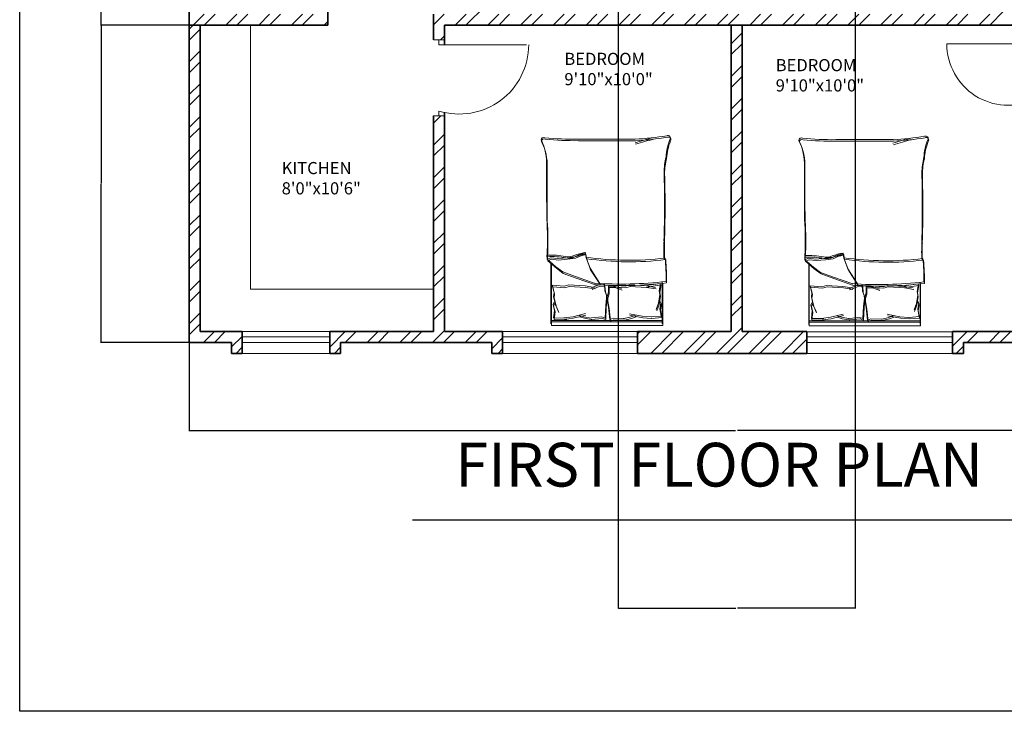
# Model space of a CAD drawing. Units: inches. Extents: x 1570 to 2186, y 1575 to 2421.
# Tile 1 of 10: x 1570 to 1975, y 1575 to 1859. Entities that reach past the tile are written whole.
import ezdxf

# ---------------------------------------------------------------- set-up
doc = ezdxf.new("R2010")
doc.units = ezdxf.units.IN
for name, color, linetype, lineweight in [('A-ANNO-DIMS', 2, 'Continuous', 18), ('A-ANNO-TTLB', 7, 'Continuous', 25), ('A-AREA-IDEN', 7, 'Continuous', 18), ('A-DOOR', 201, 'Continuous', 18), ('A-FLOR-CASE', 7, 'Continuous', 18), ('A-FURN', 8, 'Continuous', 13), ('A-GLAZ', 150, 'Continuous', 18), ('A-WALL', 7, 'Continuous', 35), ('A-WALL-PATT', 252, 'Continuous', 13)]:
    doc.layers.add(name, color=color, linetype=linetype, lineweight=lineweight)
doc.styles.get("Standard").update_dxf_attribs({"font": 'arial.ttf'})
doc.dimstyles.get("Standard").update_dxf_attribs({"dimtxt": 0.18, "dimasz": 0.18, "dimexe": 0.18, "dimexo": 0.0625, "dimgap": 0.09, "dimtad": 0, "dimtih": 1, "dimtoh": 1, "dimdec": 4, "dimzin": 0, "dimdsep": 46, "dimtxsty": 'Standard', "dimcen": 0.09, "dimadec": 0, "dimazin": 0, "dimtfac": 1, "dimtdec": 4, "dimtofl": 0, "dimtmove": 0, "dimatfit": 3, "dimfxl": 1, "dimtolj": 1, "dimtzin": 0, "dimarcsym": 0})

# ---------------------------------------------------------------- blocks, each defined once
blk = doc.blocks.new('BED-DOUBLE')
for p, q in [((3.33, 60.74), (3.33, 78.1)), ((3.33, 60.74), (3.33, 78.1)), ((3.33, 78.1), (49.16, 78.1)), ((3.55, 60.12), (3.55, 77.49)), ((3.55, 60.12), (3.55, 77.49)), ((49.16, 78.1), (49.16, 52.58)), ((49.16, 78.1), (49.16, 52.58)), ((49.38, 77.49), (49.38, 51.97)), ((49.38, 77.49), (49.38, 51.97)), ((3.33, 76.63), (49.16, 76.63)), ((3.33, 76.63), (49.16, 76.63)), ((3.55, 76.02), (49.38, 76.02)), ((3.55, 76.02), (49.38, 76.02)), ((3.74, 74.9), (7.84, 75.22)), ((3.74, 74.9), (7.84, 75.22)), ((3.74, 74.92), (4.29, 71.87)), ((3.74, 74.92), (4.29, 71.87)), ((3.95, 74.31), (4.51, 71.26)), ((3.95, 74.31), (4.51, 71.26)), ((3.96, 74.29), (8.06, 74.6)), ((3.96, 74.29), (8.06, 74.6)), ((7.84, 75.22), (7.95, 75.2)), ((7.84, 75.22), (7.95, 75.2)), ((7.95, 75.2), (11.61, 74.92)), ((7.95, 75.2), (11.61, 74.92)), ((8.06, 74.6), (8.16, 74.59)), ((8.06, 74.6), (8.16, 74.59)), ((8.16, 74.59), (11.83, 74.31)), ((8.16, 74.59), (11.83, 74.31)), ((11.61, 74.92), (16.88, 73.95)), ((11.61, 74.92), (16.88, 73.95)), ((11.83, 74.31), (17.1, 73.34)), ((11.83, 74.31), (17.1, 73.34)), ((14.25, 74.51), (16.19, 75.2)), ((14.25, 74.51), (16.19, 75.2)), ((14.46, 73.89), (16.41, 74.59)), ((14.47, 73.89), (16.41, 74.59)), ((16.19, 75.2), (18.96, 75.89)), ((16.19, 75.2), (18.96, 75.89)), ((16.41, 74.59), (19.18, 75.28)), ((16.41, 74.59), (19.18, 75.28)), ((18.96, 75.89), (19.27, 75.89)), ((18.96, 75.89), (19.27, 75.89)), ((19.18, 75.28), (19.49, 75.28)), ((19.18, 75.28), (19.49, 75.28)), ((19.27, 75.89), (23.53, 75.76)), ((19.27, 75.89), (23.53, 75.76)), ((19.49, 75.28), (23.75, 75.14)), ((19.49, 75.28), (23.75, 75.14)), ((23.53, 75.76), (24.92, 76.31)), ((23.53, 75.76), (24.92, 76.31)), ((23.75, 75.14), (25.14, 75.7)), ((23.75, 75.14), (25.14, 75.7)), ((24.92, 76.31), (25.47, 71.18)), ((24.92, 76.31), (25.47, 71.18)), ((25.14, 75.7), (25.69, 70.57)), ((25.14, 75.7), (25.69, 70.57)), ((26.83, 75.71), (26.6, 70.56)), ((26.83, 75.71), (26.6, 70.56)), ((27.05, 75.1), (26.82, 69.95)), ((27.05, 75.1), (26.82, 69.95)), ((28.25, 75.25), (26.83, 75.71)), ((28.25, 75.25), (26.83, 75.71)), ((28.47, 74.63), (27.05, 75.1)), ((28.47, 74.63), (27.05, 75.1)), ((32.49, 75.65), (28.25, 75.25)), ((32.49, 75.65), (28.25, 75.25)), ((32.71, 75.04), (28.47, 74.63)), ((32.71, 75.04), (28.47, 74.63)), ((32.8, 75.67), (32.49, 75.65)), ((32.8, 75.67), (32.49, 75.65)), ((33.02, 75.06), (32.71, 75.04)), ((33.02, 75.06), (32.71, 75.04)), ((35.61, 75.15), (32.8, 75.67)), ((35.61, 75.15), (32.8, 75.67)), ((35.83, 74.54), (33.02, 75.06)), ((35.83, 74.54), (33.02, 75.06)), ((40.2, 75.16), (35, 73.86)), ((40.2, 75.16), (35, 73.86)), ((40.42, 74.55), (35.22, 73.25)), ((40.41, 74.55), (35.22, 73.25)), ((37.59, 74.58), (35.61, 75.15)), ((37.59, 74.58), (35.61, 75.15)), ((37.81, 73.97), (35.83, 74.54)), ((37.81, 73.97), (35.83, 74.54)), ((43.84, 75.67), (40.2, 75.16)), ((43.84, 75.67), (40.2, 75.16)), ((44.06, 75.05), (40.41, 74.55)), ((44.06, 75.05), (40.42, 74.55)), ((48.06, 75.65), (42.88, 75.74)), ((42.88, 75.74), (43.84, 75.67)), ((48.06, 75.65), (42.88, 75.74)), ((42.88, 75.74), (43.84, 75.67)), ((48.28, 75.04), (43.1, 75.13)), ((43.1, 75.13), (44.06, 75.05)), ((48.28, 75.04), (43.1, 75.13)), ((43.1, 75.13), (44.06, 75.05)), ((48.06, 75.65), (47.69, 72.57)), ((48.06, 75.65), (47.69, 72.57)), ((48.28, 75.04), (47.91, 71.96)), ((48.28, 75.04), (47.91, 71.96)), ((4.29, 71.87), (3.87, 69.38)), ((4.29, 71.87), (3.87, 69.38)), ((3.87, 69.38), (4.43, 68.41)), ((3.87, 69.38), (4.43, 68.41)), ((4.51, 71.26), (4.09, 68.76)), ((4.51, 71.26), (4.09, 68.76)), ((4.29, 66.05), (4.84, 69.52)), ((4.29, 66.05), (4.84, 69.52)), ((4.51, 65.44), (5.06, 68.9)), ((4.51, 65.44), (5.06, 68.9)), ((4.84, 69.52), (5.81, 72.15)), ((4.84, 69.52), (5.81, 72.15)), ((5.06, 68.9), (6.03, 71.54)), ((5.06, 68.9), (6.03, 71.54)), ((25.47, 71.18), (26.03, 68.13)), ((25.47, 71.18), (26.03, 68.13)), ((25.69, 70.57), (26.25, 67.52)), ((25.69, 70.57), (26.25, 67.52)), ((26.6, 70.56), (26.23, 67.48)), ((26.6, 70.56), (26.23, 67.48)), ((26.82, 69.95), (26.45, 66.87)), ((26.82, 69.95), (26.45, 66.87)), ((47.29, 70.18), (46.15, 72.75)), ((47.29, 70.18), (46.16, 72.75)), ((47.51, 69.57), (46.37, 72.14)), ((47.51, 69.57), (46.37, 72.14)), ((48.06, 66.76), (47.29, 70.18)), ((48.06, 66.76), (47.29, 70.18)), ((48.28, 66.15), (47.51, 69.57)), ((48.28, 66.15), (47.51, 69.57)), ((47.69, 72.57), (48.27, 70.11)), ((47.69, 72.57), (48.26, 70.11)), ((48.27, 70.11), (47.77, 69.1)), ((48.26, 70.11), (47.77, 69.1)), ((47.91, 71.96), (48.48, 69.49)), ((47.91, 71.96), (48.48, 69.49)), ((48.48, 69.49), (47.99, 68.49)), ((48.48, 69.49), (47.99, 68.49)), ((4.09, 68.76), (4.65, 67.79)), ((4.09, 68.76), (4.65, 67.79)), ((4.57, 64.52), (4.29, 66.05)), ((4.57, 64.52), (4.29, 66.05)), ((4.79, 63.91), (4.51, 65.44)), ((4.79, 63.91), (4.51, 65.44)), ((26.03, 66.88), (25.47, 65.08)), ((26.03, 66.88), (25.47, 65.08)), ((25.47, 65.08), (25.47, 62.51)), ((25.47, 65.08), (25.47, 62.51)), ((26.25, 66.27), (25.69, 64.47)), ((26.25, 66.27), (25.69, 64.47)), ((26.03, 68.13), (26.03, 66.88)), ((26.03, 68.13), (26.03, 66.88)), ((26.23, 67.48), (26.31, 66.23)), ((26.23, 67.48), (26.31, 66.23)), ((26.25, 67.52), (26.25, 66.27)), ((26.25, 67.52), (26.25, 66.27)), ((26.31, 66.23), (26.98, 64.47)), ((26.31, 66.23), (26.98, 64.47)), ((26.45, 66.87), (26.53, 65.62)), ((26.45, 66.87), (26.53, 65.62)), ((26.53, 65.62), (27.2, 63.86)), ((26.53, 65.62), (27.2, 63.86)), ((47.88, 65.22), (48.06, 66.76)), ((47.88, 65.22), (48.06, 66.76)), ((48.62, 62.21), (47.88, 65.22)), ((48.62, 62.21), (47.88, 65.22)), ((48.09, 64.61), (48.28, 66.15)), ((48.1, 64.61), (48.28, 66.15)), ((4.01, 61.47), (4.57, 64.52)), ((4.01, 61.47), (4.57, 64.52)), ((8.9, 62.17), (4.01, 61.47)), ((8.9, 62.17), (4.01, 61.47)), ((4.23, 60.86), (4.79, 63.91)), ((4.23, 60.86), (4.79, 63.91)), ((9.12, 61.55), (4.23, 60.86)), ((9.12, 61.55), (4.23, 60.86)), ((6.12, 63.12), (9.99, 62.48)), ((6.12, 63.12), (9.99, 62.48)), ((6.34, 62.5), (10.21, 61.86)), ((6.34, 62.5), (10.21, 61.86)), ((9.99, 62.48), (8.9, 62.17)), ((9.99, 62.48), (8.9, 62.17)), ((10.21, 61.86), (9.12, 61.55)), ((10.21, 61.86), (9.12, 61.55)), ((9.99, 62.48), (16.71, 62.06)), ((9.99, 62.48), (16.71, 62.06)), ((10.21, 61.86), (16.93, 61.45)), ((10.21, 61.86), (16.93, 61.45)), ((16.71, 62.06), (18.59, 62.6)), ((16.71, 62.06), (18.59, 62.6)), ((16.93, 61.45), (18.81, 61.98)), ((16.93, 61.45), (18.81, 61.98)), ((18.59, 62.6), (23.51, 62.21)), ((18.59, 62.6), (23.51, 62.21)), ((18.81, 61.98), (23.73, 61.6)), ((18.81, 61.98), (23.73, 61.6)), ((23.12, 62.51), (20.1, 63.55)), ((23.12, 62.51), (20.1, 63.55)), ((23.33, 61.89), (20.32, 62.94)), ((23.33, 61.89), (20.32, 62.94)), ((25.47, 62.51), (23.12, 62.51)), ((25.47, 62.51), (23.12, 62.51)), ((25.69, 61.89), (23.33, 61.89)), ((25.69, 61.89), (23.33, 61.89)), ((25.69, 64.47), (25.69, 61.89)), ((25.69, 64.47), (25.69, 61.89)), ((26.98, 64.47), (27.14, 61.9)), ((26.98, 64.47), (27.14, 61.9)), ((27.14, 61.9), (29.49, 62.05)), ((27.14, 61.9), (29.49, 62.05)), ((27.2, 63.86), (27.36, 61.29)), ((27.2, 63.86), (27.36, 61.29)), ((27.36, 61.29), (29.71, 61.44)), ((27.36, 61.29), (29.71, 61.44)), ((29.02, 61.43), (33.04, 55.21)), ((29.02, 61.43), (33.04, 55.21)), ((29.24, 60.82), (33.26, 54.59)), ((29.24, 60.82), (33.26, 54.59)), ((29.49, 62.05), (32.43, 63.28)), ((29.49, 62.05), (32.43, 63.28)), ((29.71, 61.44), (32.65, 62.67)), ((29.71, 61.44), (32.65, 62.67)), ((38.98, 58.62), (30.98, 61.43)), ((38.98, 58.62), (30.98, 61.43)), ((39.2, 58.01), (31.2, 60.82)), ((39.2, 58.01), (31.2, 60.82)), ((31.23, 63.12), (35.1, 62.48)), ((31.23, 63.12), (35.1, 62.48)), ((31.45, 62.5), (35.31, 61.86)), ((31.45, 62.5), (35.31, 61.86)), ((35.1, 62.48), (41.82, 62.06)), ((35.1, 62.48), (41.82, 62.06)), ((35.31, 61.86), (42.04, 61.45)), ((35.31, 61.86), (42.04, 61.45)), ((41.82, 62.06), (43.7, 62.6)), ((41.82, 62.06), (43.7, 62.6)), ((42.04, 61.45), (43.92, 61.98)), ((42.04, 61.45), (43.92, 61.98)), ((43.7, 62.6), (48.62, 62.21)), ((43.7, 62.6), (48.62, 62.21)), ((43.92, 61.98), (48.84, 61.6)), ((43.92, 61.98), (48.84, 61.6)), ((48.84, 61.6), (48.09, 64.61)), ((48.84, 61.6), (48.1, 64.61)), ((44.32, 56.69), (38.98, 58.62)), ((44.32, 56.69), (38.98, 58.62)), ((44.54, 56.08), (39.2, 58.01)), ((44.54, 56.08), (39.2, 58.01)), ((33.04, 55.21), (34.67, 50.9)), ((33.04, 55.21), (34.67, 50.9)), ((33.26, 54.59), (34.89, 50.29)), ((33.26, 54.59), (34.89, 50.29)), ((47.15, 54.61), (44.32, 56.69)), ((47.15, 54.61), (44.32, 56.69)), ((47.37, 54), (44.54, 56.08)), ((47.37, 54), (44.54, 56.08)), ((50.7, 51.5), (47.15, 54.61)), ((50.7, 51.5), (47.15, 54.61)), ((50.92, 50.88), (47.37, 54)), ((50.92, 50.88), (47.37, 54)), ((34.67, 50.9), (34.97, 48.97)), ((34.67, 50.9), (34.97, 48.97)), ((34.89, 50.29), (35.19, 48.36)), ((34.89, 50.29), (35.19, 48.36)), ((34.97, 48.97), (37.34, 49.57)), ((34.97, 48.97), (37.34, 49.57)), ((35.19, 48.36), (37.56, 48.95)), ((35.19, 48.36), (37.56, 48.95)), ((37.34, 49.57), (39.27, 50.46)), ((37.34, 49.57), (39.27, 50.46)), ((37.56, 48.95), (39.49, 49.84)), ((37.56, 48.95), (39.49, 49.84)), ((39.27, 50.46), (42.54, 50.9)), ((39.27, 50.46), (42.54, 50.9)), ((39.49, 49.84), (42.76, 50.29)), ((39.49, 49.84), (42.76, 50.29)), ((42.54, 50.9), (46.26, 51.2)), ((42.54, 50.9), (46.26, 51.2)), ((42.76, 50.29), (46.47, 50.59)), ((42.76, 50.29), (46.47, 50.59)), ((46.26, 51.2), (49.23, 50.9)), ((46.26, 51.2), (49.23, 50.9)), ((46.47, 50.59), (49.45, 50.29)), ((46.47, 50.59), (49.44, 50.29)), ((49.23, 50.9), (50.7, 51.5)), ((49.23, 50.9), (50.7, 51.5)), ((49.44, 50.29), (50.92, 50.88)), ((49.45, 50.29), (50.92, 50.88)), ((50.78, 49.82), (50.7, 51.5, 3.71)), ((50.78, 49.82), (50.7, 51.5, 3.71)), ((51, 49.21), (50.92, 50.88, 3.71)), ((51, 49.21), (50.92, 50.88, 3.71)), ((14.45, 2.11), (38.05, 2.11)), ((14.45, 2.11), (38.05, 2.11)), ((14.66, 1.49), (38.27, 1.49)), ((14.67, 1.49), (38.27, 1.49))]:
    blk.add_line(p, q)
for centre, radius, start, end in [((20.48, -96.48), 158.2, 86.0865, 96.7821), ((20.48, -96.48), 158.2, 86.0865, 96.7821), ((20.7, -97.1), 158.2, 86.0865, 96.7821), ((20.7, -97.1), 158.2, 86.0865, 96.7821), ((81.67, 58.83), 79.89, 178.7218, 185.604), ((81.67, 58.83), 79.89, 178.7218, 185.604), ((81.89, 58.22), 79.89, 178.7218, 185.604), ((81.89, 58.22), 79.89, 178.7218, 185.604), ((17.03, -71.8), 123.73, 81.7845, 96.9006), ((17.03, -71.8), 123.73, 81.7845, 96.9006), ((17.25, -72.42), 123.73, 81.7845, 96.9006), ((17.25, -72.42), 123.73, 81.7845, 96.9006), ((-160.45, 48.21), 163.13, 358.4762, 1.0082), ((-160.45, 48.21), 163.13, 358.4762, 1.0082), ((-160.23, 47.59), 163.13, 358.4762, 1.0082), ((-160.23, 47.59), 163.13, 358.4762, 1.0082), ((35.13, 48.91), 0.177, 160.2464, 271.1377), ((35.13, 48.91), 0.177, 160.2464, 271.1377), ((29.88, 76.68), 28.44, 280.6617, 289.8806), ((29.88, 76.68), 28.44, 280.6617, 289.8806), ((30.1, 76.07), 28.44, 280.6617, 289.8806), ((30.1, 76.07), 28.44, 280.6617, 289.8806), ((41.95, 44.48), 5.97, 78.6608, 113.7384), ((41.95, 44.48), 5.97, 78.6608, 113.7384), ((42.17, 43.86), 5.97, 78.6608, 113.7384), ((42.17, 43.86), 5.97, 78.6608, 113.7384), ((49.22, 84.49), 34.7, 259.8763, 272.5657), ((49.22, 84.49), 34.7, 259.8763, 272.5657), ((49.44, 83.87), 34.7, 259.8763, 272.5657), ((49.44, 83.87), 34.7, 259.8763, 272.5657), ((174.79, 43.28), 124.19, 176.9791, 183.8365), ((174.79, 43.28), 124.19, 176.9791, 183.8365), ((175.01, 42.66), 124.19, 176.9791, 183.8365), ((175.01, 42.66), 124.19, 176.9791, 183.8365), ((35.35, 48.3), 0.177, 160.2464, 271.1377), ((35.35, 48.3), 0.177, 160.2464, 271.1377), ((464.94, 29.56), 462.53, 178.2277, 181.7185), ((464.94, 29.56), 462.53, 178.2277, 181.7185), ((465.16, 28.95), 462.53, 178.2277, 181.7185), ((465.16, 28.95), 462.53, 178.2277, 181.7185), ((-4323.86, 13.06), 4374.8, 0.00217, 0.28689), ((-4323.86, 13.06), 4374.8, 0.00217, 0.28689), ((-4323.64, 12.45), 4374.8, 0.00217, 0.28689), ((-4323.64, 12.45), 4374.8, 0.00217, 0.28689), ((-25.8, 16.23), 28.42, 346.0648, 358.9113), ((-25.8, 16.23), 28.42, 346.0648, 358.9113), ((-25.58, 15.62), 28.42, 346.0648, 358.9113), ((-25.58, 15.62), 28.42, 346.0648, 358.9113), ((73.03, 12.25), 22.12, 177.4714, 206.4681), ((73.03, 12.25), 22.12, 177.4714, 206.4681), ((73.25, 11.64), 22.12, 177.4714, 206.4681), ((73.25, 11.64), 22.12, 177.4714, 206.4681), ((-20.77, 10.71), 22.6, 337.9751, 356.652), ((-20.77, 10.71), 22.6, 337.9751, 356.652), ((-20.55, 10.1), 22.6, 337.9751, 356.652), ((-20.55, 10.1), 22.6, 337.9751, 356.652), ((1.04, 1.65), 1.04, 146.1736, 293.4781), ((1.04, 1.65), 1.04, 146.1736, 293.4781), ((1.26, 1.04), 1.04, 146.1736, 293.4781), ((1.26, 1.04), 1.04, 146.1736, 293.4781), ((20.55, -114.5), 116.77, 92.9958, 99.4091), ((20.55, -114.5), 116.77, 92.9958, 99.4091), ((20.77, -115.11), 116.77, 92.9958, 99.4091), ((20.77, -115.11), 116.77, 92.9958, 99.4091), ((-16.52, 100.84), 102.09, 283.3832, 287.7053), ((-16.52, 100.84), 102.09, 283.3832, 287.7053), ((-16.3, 100.23), 102.09, 283.3832, 287.7053), ((-16.3, 100.23), 102.09, 283.3832, 287.7053), ((39.46, -125.47), 127.58, 84.4998, 90.6351), ((39.46, -125.47), 127.58, 84.4998, 90.6351), ((39.68, -126.08), 127.58, 84.4998, 90.6351), ((39.68, -126.08), 127.58, 84.4998, 90.6351), ((52.18, 2.47), 1.06, 242.6588, 356.02), ((52.18, 2.47), 1.06, 242.6588, 356.02), ((52.4, 1.85), 1.06, 242.6588, 356.02), ((52.4, 1.85), 1.06, 242.6588, 356.02)]:
    blk.add_arc(centre, radius, start, end)
blk = doc.blocks.new('*D31')
at = {"layer": 'A-ANNO-DIMS', "color": 0, "lineweight": -2, "transparency": 16777216}
for p, q in [((1639.59, 1726.19), (1639.59, 1689.77)), ((2090.09, 1726.19), (2090.09, 1689.77)), ((1639.77, 1689.95), (1864.44, 1689.95)), ((2089.91, 1689.95), (1865.24, 1689.95))]:
    blk.add_line(p, q, dxfattribs=at)
at = {"layer": 'A-ANNO-DIMS', "color": 0, "transparency": 16777216}
for points in [[(1639.77, 1689.98), (1639.77, 1689.92), (1639.59, 1689.95)], [(2089.91, 1689.98), (2089.91, 1689.92), (2090.09, 1689.95)]]:
    blk.add_solid(points, dxfattribs=at)
at = {"layer": 'Defpoints', "color": 0, "transparency": 16777216}
for p in [(1639.59, 1726.25), (2090.09, 1726.25), (1639.59, 1689.95)]:
    blk.add_point(p, dxfattribs=at)
at = {"layer": 'A-ANNO-DIMS', "color": 0, "transparency": 16777216, "insert": (1864.84, 1689.95), "char_height": 0.18, "attachment_point": 5}
blk.add_mtext('\\A1;450.5', dxfattribs=at)
blk = doc.blocks.new('*D33')
at = {"layer": 'A-ANNO-DIMS', "color": 0, "lineweight": -2, "transparency": 16777216}
for p, q in [((1639.53, 1856.75), (1603.11, 1856.75)), ((1603.29, 1856.57), (1603.29, 1791.68)), ((1603.29, 1726.43), (1603.29, 1791.32)), ((1639.53, 1726.25), (1603.11, 1726.25))]:
    blk.add_line(p, q, dxfattribs=at)
at = {"layer": 'A-ANNO-DIMS', "color": 0, "transparency": 16777216}
for points in [[(1603.26, 1856.57), (1603.32, 1856.57), (1603.29, 1856.75)], [(1603.26, 1726.43), (1603.32, 1726.43), (1603.29, 1726.25)]]:
    blk.add_solid(points, dxfattribs=at)
at = {"layer": 'Defpoints', "color": 0, "transparency": 16777216}
for p in [(1603.29, 1856.75), (1639.59, 1856.75), (1639.59, 1726.25)]:
    blk.add_point(p, dxfattribs=at)
at = {"layer": 'A-ANNO-DIMS', "color": 0, "transparency": 16777216, "insert": (1603.29, 1791.5), "char_height": 0.18, "attachment_point": 5}
blk.add_mtext('\\A1;130.5', dxfattribs=at)
blk = doc.blocks.new('*D34')
at = {"layer": 'A-ANNO-DIMS', "color": 0, "lineweight": -2, "transparency": 16777216}
for p, q in [((1639.53, 1913.75), (1603.11, 1913.75)), ((1603.29, 1913.57), (1603.29, 1885.43)), ((1603.29, 1856.93), (1603.29, 1885.07)), ((1639.53, 1856.75), (1603.11, 1856.75))]:
    blk.add_line(p, q, dxfattribs=at)
at = {"layer": 'A-ANNO-DIMS', "color": 0, "transparency": 16777216}
for points in [[(1603.26, 1913.57), (1603.32, 1913.57), (1603.29, 1913.75)], [(1603.26, 1856.93), (1603.32, 1856.93), (1603.29, 1856.75)]]:
    blk.add_solid(points, dxfattribs=at)
at = {"layer": 'Defpoints', "color": 0, "transparency": 16777216}
for p in [(1603.29, 1913.75), (1639.59, 1913.75), (1639.59, 1856.75)]:
    blk.add_point(p, dxfattribs=at)
at = {"layer": 'A-ANNO-DIMS', "color": 0, "transparency": 16777216, "insert": (1603.29, 1885.25), "char_height": 0.18, "attachment_point": 5}
blk.add_mtext('\\A1;57', dxfattribs=at)
blk = doc.blocks.new('*D39')
at = {"layer": 'A-ANNO-DIMS', "color": 0, "lineweight": -2, "transparency": 16777216}
for p, q in [((1816.09, 2097.8), (1816.09, 1616.73)), ((1913.59, 2097.8), (1913.59, 1616.73)), ((1816.27, 1616.91), (1864.51, 1616.91)), ((1913.41, 1616.91), (1865.16, 1616.91))]:
    blk.add_line(p, q, dxfattribs=at)
at = {"layer": 'A-ANNO-DIMS', "color": 0, "transparency": 16777216}
for points in [[(1816.27, 1616.94), (1816.27, 1616.88), (1816.09, 1616.91)], [(1913.41, 1616.94), (1913.41, 1616.88), (1913.59, 1616.91)]]:
    blk.add_solid(points, dxfattribs=at)
at = {"layer": 'Defpoints', "color": 0, "transparency": 16777216}
for p in [(1816.09, 2097.86), (1913.59, 2097.86), (1913.59, 1616.91)]:
    blk.add_point(p, dxfattribs=at)
at = {"layer": 'A-ANNO-DIMS', "color": 0, "transparency": 16777216, "insert": (1864.84, 1616.91), "char_height": 0.18, "attachment_point": 5}
blk.add_mtext('\\A1;97.5', dxfattribs=at)

msp = doc.modelspace()

# ---------------------------------------------------------------- hatches: boundary and pattern name
at = {"layer": 'A-WALL-PATT'}
h = msp.add_hatch(dxfattribs=at)
h.set_pattern_fill('ANSI32', color=256)
h.paths.add_polyline_path([(1762.0975, 2362.1492), (1757.5975, 2362.1492), (1757.5975, 2357.6492), (1709.1163, 2357.6492), (1709.1163, 2362.1492), (1704.6163, 2362.1492), (1704.6163, 2353.1492), (1740.0886, 2353.1492), (1740.0886, 2261.8115), (1744.5886, 2261.8115), (1744.5886, 2353.1492), (1762.0975, 2353.1492)])
h.paths.add_polyline_path([(1890.2592, 2362.1492), (1885.7592, 2362.1492), (1826.5975, 2362.1492), (1822.0975, 2362.1492), (1822.0975, 2353.1492), (1862.5886, 2353.1492), (1862.5886, 2227.1492), (1744.5886, 2227.1492), (1744.5886, 2229.5389), (1742.3386, 2229.5389), (1740.0886, 2229.5389), (1740.0886, 2222.6492), (1744.5886, 2222.6492), (1756.186, 2222.6492), (1756.186, 2216.3571), (1760.686, 2216.3571), (1760.686, 2222.6492), (1832.686, 2222.6492), (1832.686, 2212.5994), (1837.186, 2212.5994), (1837.186, 2222.6492), (1893.186, 2222.6492), (1893.186, 2212.5994), (1897.686, 2212.5994), (1897.686, 2222.6492), (1989.5886, 2222.6492), (1989.5886, 2227.1492), (1989.5886, 2232.6585), (1987.3386, 2232.6585), (1985.0886, 2232.6585), (1985.0886, 2227.1492), (1867.0886, 2227.1492), (1867.0886, 2353.1492), (1890.2592, 2353.1492)])
h.paths.add_polyline_path([(1644.0886, 2353.1492), (1668.6163, 2353.1492), (1668.6163, 2362.1492), (1664.1163, 2362.1492), (1664.1163, 2358.9932), (1664.1163, 2357.6492), (1639.5886, 2357.6492), (1639.5886, 2213.8746), (1644.0886, 2213.8746), (1644.0886, 2222.6492), (1692.0886, 2222.6492), (1692.0886, 2215.9343), (1696.5886, 2215.9343), (1696.5886, 2222.6492), (1696.5886, 2227.1492), (1644.0886, 2227.1492)])
h.paths.add_polyline_path([(2013.0435, 2362.1492), (2008.5435, 2362.1492), (2008.5435, 2357.6492), (1954.7592, 2357.6492), (1954.7592, 2362.1492), (1950.2592, 2362.1492), (1950.2592, 2353.1492), (1985.0886, 2353.1492), (1985.0886, 2260.8534), (1989.5886, 2260.8534), (1989.5886, 2353.1492), (2013.0435, 2353.1492)])
h.paths.add_polyline_path([(2090.0886, 2357.6492), (2053.5435, 2357.6492), (2053.5435, 2362.1492), (2049.0435, 2362.1492), (2049.0435, 2353.1492), (2085.5886, 2353.1492), (2085.5886, 2227.1492), (2033.0886, 2227.1492), (2033.0886, 2222.6492), (2033.0886, 2214.4464), (2037.5886, 2214.4464), (2037.5886, 2222.6492), (2085.5886, 2222.6492), (2085.5886, 2212.4409), (2090.0886, 2212.4409)])
h.paths.add_polyline_path([(2090.0886, 2188.4409), (2087.8386, 2188.4409), (2085.5886, 2188.4409), (2085.5886, 2180.6492), (2037.5886, 2180.6492), (2037.5886, 2196.7956), (2033.0886, 2196.7956), (2033.0886, 2176.1492), (2037.5886, 2176.1492), (2045.0886, 2176.1492), (2045.0886, 2169.8988), (2049.5886, 2169.8988), (2049.5886, 2176.1492), (2085.5886, 2176.1492), (2085.5886, 2167.785), (2090.0886, 2167.785)])
h.paths.add_polyline_path([(2049.5886, 2147.4502), (2047.3386, 2147.4502), (2045.0886, 2147.4502), (2045.0886, 2124.4703), (2049.5886, 2124.4703)])
h.paths.add_polyline_path([(2090.0886, 2047.1492), (2049.5886, 2047.1492), (2049.5886, 2064.4703), (2045.0886, 2064.4703), (2045.0886, 2047.1492), (1918.0886, 2047.1492), (1918.0886, 2051.2061), (1913.5886, 2051.2061), (1913.5886, 2047.1492), (1913.5886, 2036.6872), (1918.0886, 2036.6872), (1918.0886, 2042.7492), (2045.0886, 2042.7492), (2045.0886, 2027.0686), (2049.5886, 2027.0686), (2049.5886, 2042.7492), (2090.0886, 2042.7492)])
h.paths.add_polyline_path([(1918.0886, 2005.9338), (1915.8386, 2005.9338), (1913.5886, 2005.9338), (1913.5886, 1913.7492), (1918.0886, 1913.7492)])
h.paths.add_polyline_path([(2090.0886, 1913.7492), (2049.5886, 1913.7492), (2045.0886, 1913.7492), (2033.0886, 1913.7492), (2033.0886, 1909.2492), (2033.0886, 1900.9803), (2037.5886, 1900.9803), (2037.5886, 1909.2492), (2085.5886, 1909.2492), (2085.5886, 1861.2492), (2037.5886, 1861.2492), (2037.5886, 1880.0859), (2033.0886, 1880.0859), (2033.0886, 1856.7492), (2085.5886, 1856.7492), (2085.5886, 1730.7492), (2054.2483, 1730.7492), (2054.2483, 1721.7492), (2058.7483, 1721.7492), (2058.7483, 1726.2492), (2090.0886, 1726.2492)])
h.paths.add_polyline_path([(2049.5886, 1967.0686), (2045.0886, 1967.0686), (2045.0886, 1913.7492), (2049.5886, 1913.7492)])
h.paths.add_polyline_path([(1989.5886, 1824.1695), (1987.3386, 1824.1695), (1985.0886, 1824.1695), (1985.0886, 1730.7492), (1989.5886, 1730.7492)])
h.paths.add_polyline_path([(1989.5886, 1861.2492), (1974.9963, 1861.2492), (1974.9963, 1865.9306), (1972.7463, 1865.9306), (1970.4963, 1865.9306), (1970.4963, 1861.2492), (1898.4963, 1861.2492), (1898.4963, 1874.2999), (1893.9963, 1874.2999), (1893.9963, 1861.2492), (1890.5886, 1861.2492), (1837.9963, 1861.2492), (1837.9963, 1874.3159), (1833.4963, 1874.3159), (1833.4963, 1861.2492), (1761.4963, 1861.2492), (1761.4963, 1865.0209), (1759.2463, 1865.0209), (1756.9963, 1865.0209), (1756.9963, 1861.2492), (1740.0886, 1861.2492), (1740.0886, 1856.7492), (1740.0886, 1850.7206), (1744.5886, 1850.7206), (1744.5886, 1856.7492), (1985.0886, 1856.7492), (1985.0886, 1851.0804), (1989.5886, 1851.0804), (1989.5886, 1856.7492)])
h.paths.add_polyline_path([(1989.5886, 1913.7492), (1740.0886, 1913.7492), (1740.0886, 1909.2492), (1756.9963, 1909.2492), (1756.9963, 1890.279), (1761.4963, 1890.279), (1761.4963, 1909.2492), (1833.4963, 1909.2492), (1833.4963, 1898.3159), (1837.9963, 1898.3159), (1837.9963, 1909.2492), (1890.5886, 1909.2492), (1893.9963, 1909.2492), (1893.9963, 1898.2999), (1898.4963, 1898.2999), (1898.4963, 1909.2492), (1970.4963, 1909.2492), (1970.4963, 1886.9887), (1974.9963, 1886.9887), (1974.9963, 1909.2492), (1989.5886, 1909.2492)])
h.paths.add_polyline_path([(1893.7344, 1730.7492), (1867.0886, 1730.7492), (1867.0886, 1856.7492), (1862.5886, 1856.7492), (1862.5886, 1730.7492), (1824.0492, 1730.7492), (1824.0492, 1721.7492), (1893.7344, 1721.7492)])
h.paths.add_polyline_path([(2018.2483, 1730.7492), (1953.7344, 1730.7492), (1953.7344, 1721.7492), (1958.2344, 1721.7492), (1958.2344, 1726.2492), (2013.7483, 1726.2492), (2013.7483, 1721.7492), (2018.2483, 1721.7492)])
h.paths.add_polyline_path([(1768.5492, 1730.7492), (1764.0492, 1730.7492), (1744.5886, 1730.7492), (1744.5886, 1819.4364), (1742.3386, 1819.4364), (1740.0886, 1819.4364), (1740.0886, 1730.7492), (1697.3801, 1730.7492), (1697.3801, 1721.7492), (1701.8801, 1721.7492), (1701.8801, 1726.2492), (1764.0492, 1726.2492), (1764.0492, 1721.7492), (1768.5492, 1721.7492)])
h.paths.add_polyline_path([(1644.0886, 1856.7492), (1639.5886, 1856.7492), (1639.5886, 1726.2492), (1657.0315, 1726.2492), (1657.0315, 1721.7492), (1661.3801, 1721.7492), (1661.3801, 1730.7492), (1644.0886, 1730.7492)])
h.paths.add_polyline_path([(1696.5886, 1876.1809), (1692.0886, 1876.1809), (1692.0886, 1861.2492), (1684.5886, 1861.2492), (1644.0886, 1861.2492), (1644.0886, 1909.2492), (1692.0886, 1909.2492), (1692.0886, 1900.3394), (1696.5886, 1900.3394), (1696.5886, 1913.7492), (1684.5886, 1913.7492), (1684.5886, 1920.2115), (1682.3386, 1920.2115), (1680.0886, 1920.2115), (1680.0886, 1913.7492), (1639.5886, 1913.7492), (1639.5886, 1856.7492), (1684.5886, 1856.7492), (1692.0886, 1856.7492), (1696.5886, 1856.7492)])
h.paths.add_polyline_path([(1684.5886, 2042.7492), (1811.5886, 2042.7492), (1811.5886, 2038.2991), (1816.0886, 2038.2991), (1816.0886, 2042.7492), (1816.0886, 2052.5708), (1813.8386, 2052.5708), (1811.5886, 2052.5708), (1811.5886, 2047.1492), (1684.5886, 2047.1492), (1684.5886, 2064.4703), (1680.0886, 2064.4703), (1680.0886, 2047.1492), (1639.5886, 2047.1492), (1639.5886, 2042.7492), (1680.0886, 2042.7492), (1680.0886, 2024.0762), (1684.5886, 2024.0762)])
h.paths.add_polyline_path([(1684.5886, 1964.0762), (1680.0886, 1964.0762), (1680.0886, 1944.6145), (1684.5886, 1944.6145)])
h.paths.add_polyline_path([(1816.0886, 1973.7492), (1876.0886, 1973.7492), (1876.0886, 1959.17), (1880.5886, 1959.17), (1880.5886, 1973.7492), (1880.5886, 1978.2492), (1816.0886, 1978.2492), (1816.0886, 2005.9338), (1813.8386, 2005.9338), (1811.5886, 2005.9338), (1811.5886, 1913.7492), (1816.0886, 1913.7492)])
h.paths.add_polyline_path([(1837.186, 2180.6492), (1837.186, 2188.5994), (1834.936, 2188.5994), (1832.686, 2188.5994), (1832.686, 2180.6492), (1760.686, 2180.6492), (1760.686, 2197.4807), (1756.186, 2197.4807), (1756.186, 2180.6492), (1744.5886, 2180.6492), (1740.0886, 2180.6492), (1740.0886, 2176.1492), (1837.186, 2176.1492)])
h.paths.add_polyline_path([(1974.186, 2196.8744), (1971.936, 2196.8744), (1969.686, 2196.8744), (1969.686, 2180.6492), (1897.686, 2180.6492), (1897.686, 2188.5994), (1895.436, 2188.5994), (1893.186, 2188.5994), (1893.186, 2180.6492), (1893.186, 2176.1492), (1974.186, 2176.1492)])
h.paths.add_polyline_path([(1918.0886, 2176.1492), (1913.5886, 2176.1492), (1913.5886, 2081.3709), (1918.0886, 2081.3709)])
h.paths.add_polyline_path([(1816.0886, 2176.1492), (1811.5886, 2176.1492), (1811.5886, 2081.3709), (1816.0886, 2081.3709)])
h.paths.add_polyline_path([(1684.5886, 2150.4939), (1682.3386, 2150.4939), (1680.0886, 2150.4939), (1680.0886, 2124.4703), (1684.5886, 2124.4703)])
h.paths.add_polyline_path([(1696.5886, 2180.6492), (1696.5886, 2197.4701), (1692.0886, 2197.4701), (1692.0886, 2180.6492), (1644.0886, 2180.6492), (1644.0886, 2189.8746), (1641.8386, 2189.8746), (1639.5886, 2189.8746), (1639.5886, 2169.814), (1644.0886, 2169.814), (1644.0886, 2176.1492), (1680.0886, 2176.1492), (1680.0886, 2171.7002), (1684.5886, 2171.7002), (1684.5886, 2176.1492), (1696.5886, 2176.1492)])

# ---------------------------------------------------------------- linework, layer by layer
at = {"layer": 'A-ANNO-TTLB'}
msp.add_line((1731.492, 1653.2104), (2001.1233, 1653.2104), dxfattribs=at)
msp.add_lwpolyline([(1569.8198, 2421.0436), (2186.3437, 2421.0436), (2186.3437, 1574.5084), (1569.8198, 1574.5084)], close=True, dxfattribs=at)
at = {"layer": 'A-DOOR'}
for p, q in [((1740.0886, 1850.7206), (1744.5886, 1850.7206)), ((1744.5886, 1850.7206), (1742.3386, 1850.7206)), ((1742.3386, 1850.7206), (1742.3386, 1848.7206)), ((1742.3386, 1848.7206), (1778.3386, 1848.7206)), ((1987.3386, 1849.0804), (1951.3386, 1849.0804)), ((1740.0886, 1819.4364), (1744.5886, 1819.4364)), ((1742.3386, 1819.4364), (1742.3386, 1821.4364)), ((1744.5886, 1819.4364), (1742.3386, 1819.4364))]:
    msp.add_line(p, q, dxfattribs=at)
for centre, radius, start, end in [((1750.7294, 1848.7206), 28.5453, 252.905619, 0), ((1976.629, 1849.0804), 25.2904, 180, 295.053575)]:
    msp.add_arc(centre, radius, start, end, dxfattribs=at)
at = {"layer": 'A-FLOR-CASE'}
for p, q in [((1664.8545, 1856.7492), (1664.8545, 1748.1877)), ((1664.8545, 1748.1877), (1740.0886, 1748.1877))]:
    msp.add_line(p, q, dxfattribs=at)
at = {"layer": 'A-GLAZ'}
for p, q in [((1661.3801, 1730.7492), (1697.3801, 1730.7492)), ((1824.0492, 1730.7492), (1768.5492, 1730.7492)), ((1893.7344, 1730.6363), (1953.7344, 1730.6363)), ((1697.3801, 1728.6054), (1661.3801, 1728.6054)), ((1661.3801, 1726.2492), (1697.3801, 1726.2492)), ((1824.0492, 1728.5321), (1768.5492, 1728.5321)), ((1768.5492, 1726.2492), (1824.0492, 1726.2492)), ((1953.7344, 1728.5582), (1893.7344, 1728.5582)), ((1893.7344, 1726.2492), (1953.7344, 1726.2492)), ((1661.3801, 1721.7492), (1697.3801, 1721.7492)), ((1768.5492, 1721.7492), (1824.0492, 1721.7492)), ((1893.7344, 1721.7492), (1953.7344, 1721.7492))]:
    msp.add_line(p, q, dxfattribs=at)
at = {"layer": 'A-WALL'}
for p, q in [((1639.5886, 1913.7492), (1639.5886, 1726.2492)), ((1696.5886, 1856.7492), (1696.5886, 1876.1809)), ((1740.0886, 1861.2492), (1740.0886, 1856.7492)), ((1684.5886, 1856.7492), (1639.5886, 1856.7492)), ((1644.0886, 1856.7492), (1644.0886, 1730.7492)), ((1684.5886, 1856.7492), (1692.0886, 1856.7492)), ((1692.0886, 1856.7492), (1696.5886, 1856.7492)), ((1740.0886, 1856.7492), (1740.0886, 1850.7206)), ((1744.5886, 1856.7492), (1744.5886, 1848.7206)), ((1985.0886, 1856.7492), (1744.5886, 1856.7492)), ((1862.5886, 1856.7492), (1862.5886, 1730.7492)), ((1867.0886, 1856.7492), (1867.0886, 1730.7492)), ((1740.0886, 1819.4364), (1740.0886, 1730.7492)), ((1744.5886, 1820.8437), (1744.5886, 1730.7492)), ((1661.3801, 1730.7492), (1644.0886, 1730.7492)), ((1661.3801, 1730.7492), (1661.3801, 1721.7492)), ((1697.3801, 1721.7492), (1697.3801, 1730.7492)), ((1740.0886, 1730.7492), (1697.3801, 1730.7492)), ((1764.0492, 1730.7492), (1744.5886, 1730.7492)), ((1764.0492, 1730.7492), (1768.5492, 1730.7492)), ((1768.5492, 1730.7492), (1768.5492, 1721.7492)), ((1824.0492, 1721.7492), (1824.0492, 1730.7492)), ((1862.5886, 1730.7492), (1824.0492, 1730.7492)), ((1893.7344, 1730.7492), (1867.0886, 1730.7492)), ((1893.7344, 1730.7492), (1893.7344, 1721.7492)), ((1953.7344, 1721.7492), (1953.7344, 1730.7492)), ((2018.2483, 1730.7492), (1953.7344, 1730.7492)), ((1657.0315, 1726.2492), (1639.5886, 1726.2492)), ((1657.0315, 1726.2492), (1657.0315, 1721.7492)), ((1701.8801, 1721.7492), (1701.8801, 1726.2492)), ((1764.0492, 1726.2492), (1701.8801, 1726.2492)), ((1764.0492, 1726.2492), (1764.0492, 1721.7492)), ((1958.2344, 1721.7492), (1958.2344, 1726.2492)), ((2013.7483, 1726.2492), (1958.2344, 1726.2492)), ((1661.3801, 1721.7492), (1657.0315, 1721.7492)), ((1697.3801, 1721.7492), (1701.8801, 1721.7492)), ((1701.8801, 1721.7492), (1697.3801, 1721.7492)), ((1768.5492, 1721.7492), (1764.0492, 1721.7492)), ((1893.7344, 1721.7492), (1824.0492, 1721.7492)), ((1893.7344, 1721.7492), (1889.2344, 1721.7492)), ((1953.7344, 1721.7492), (1958.2344, 1721.7492)), ((1958.2344, 1721.7492), (1953.7344, 1721.7492))]:
    msp.add_line(p, q, dxfattribs=at)

# ---------------------------------------------------------------- block references
at = {"layer": 'A-FURN', "rotation": 180}
for p in [(1837.8068, 1811.3434), (1943.8887, 1811.1493)]:
    msp.add_blockref('BED-DOUBLE', p, dxfattribs=at)

# ---------------------------------------------------------------- texts
at = {"layer": 'A-ANNO-TTLB', "insert": (1749.0635, 1684.9505), "char_height": 18, "attachment_point": 1}
msp.add_mtext_dynamic_manual_height_columns('FIRST FLOOR PLAN ', width=635.239319, gutter_width=12.5, heights=[0], dxfattribs=at)
at = {"layer": 'A-AREA-IDEN', "char_height": 5, "attachment_point": 1}
for s, width, insert in [('BEDROOM\\P9\'10"x10\'0"', 115.917113, (1793.9525, 1845.3843)), ('BEDROOM\\P9\'10"x10\'0"', 141.163472, (1880.9155, 1842.8001)), ('KITCHEN\\P8\'0"x10\'6"', 206.367623, (1677.625, 1800.4703))]:
    msp.add_mtext_dynamic_manual_height_columns(s, width=width, gutter_width=12.5, heights=[0], dxfattribs=dict(at, insert=insert))

# ---------------------------------------------------------------- dimensions: what is measured, and where the dimension line sits
at = {"layer": 'A-ANNO-DIMS'}
dim = msp.add_linear_dim(base=(1913.5886, 1616.9104), p1=(1816.0886, 2097.8597), p2=(1913.5886, 2097.8597), dimstyle='Standard', override={"dimdec": 1, "dimlfac": 1, "dimrnd": 0, "dimzin": 0, "dimdsep": 46, "dimlunit": 2}, dxfattribs=at)
dim.commit()
dim.dimension.update_dxf_attribs({"geometry": '*D39', "text_midpoint": (1864.8386, 1616.9104)})
for base, p1, p2, angle, override, picture, middle in [((1603.2886, 1913.7492), (1639.5886, 1856.7492), (1639.5886, 1913.7492), 90, {"dimdec": 0, "dimlfac": 1, "dimrnd": 0, "dimzin": 0, "dimdsep": 46, "dimlunit": 2}, '*D34', (1603.2886, 1885.2492)), ((1603.2886, 1856.7492), (1639.5886, 1726.2492), (1639.5886, 1856.7492), 90, {"dimdec": 1, "dimlfac": 1, "dimrnd": 0, "dimzin": 0, "dimdsep": 46, "dimlunit": 2}, '*D33', (1603.2886, 1791.4992)), ((1639.5886, 1689.9492), (2090.0886, 1726.2492), (1639.5886, 1726.2492), 180, {"dimdec": 1, "dimlfac": 1, "dimrnd": 0, "dimzin": 0, "dimdsep": 46, "dimlunit": 2}, '*D31', (1864.8386, 1689.9492))]:
    dim = msp.add_linear_dim(base=base, p1=p1, p2=p2, angle=angle, dimstyle='Standard', override=override, dxfattribs=at)
    dim.commit()
    dim.dimension.update_dxf_attribs({"geometry": picture, "text_midpoint": middle})

doc.saveas('drawing.dxf')
